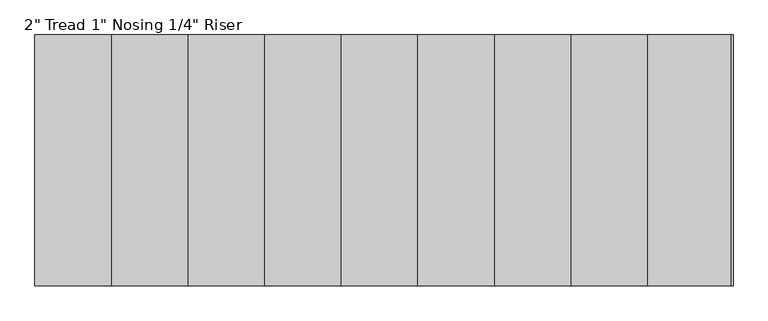
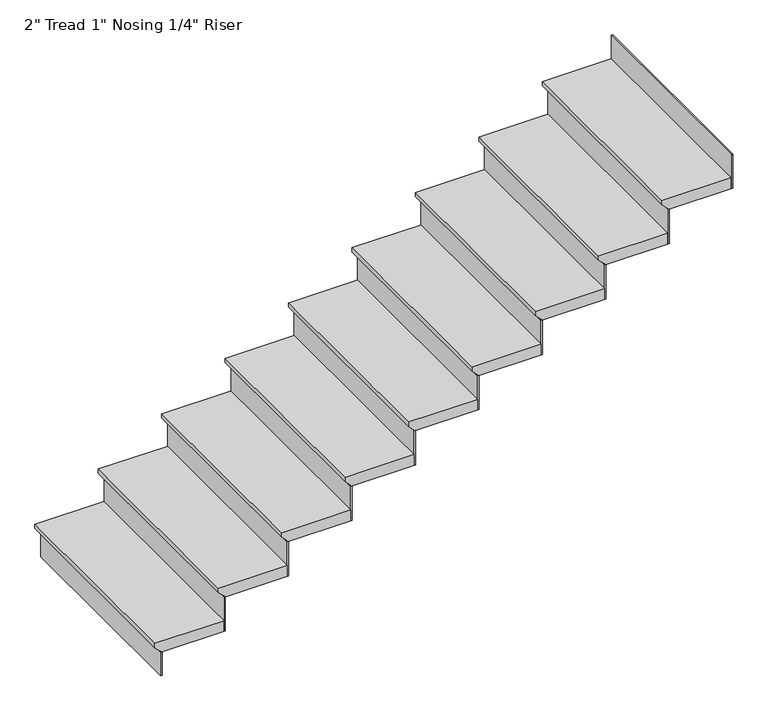
"""IFC4 building model written with IfcOpenShell, lengths in millimetres: stair flight geometry."""

from ifc_helpers import new_model, si_unit, origin, place, context, project, spatial, faceted_brep, source, transform, mapped, element, save


def stair_flight_54a58d27(model_context):
    return source(origin(), model_context, "Body", "Brep", [
        faceted_brep([(-1591.1154463, -4737.3544725, 3341.37), (-1591.1154463, -4737.3544725, 3360.42), (-1591.1154463, -3822.9544725, 3360.42), (-1591.1154463, -3822.9544725, 3341.37), (-1565.7154463, -4737.3544725, 3315.97), (-1565.7154463, -3822.9544725, 3315.97), (-1286.3154463, -4737.3544725, 3360.42), (-1286.3154463, -3822.9544725, 3360.42), (-1565.7154463, -3822.9544725, 3309.62), (-1286.3154463, -3822.9544725, 3309.62), (-1286.3154463, -4737.3544725, 3309.62), (-1565.7154463, -4737.3544725, 3309.62)], [[[0, 1, 2, 3]], [[4, 0, 3, 5]], [[2, 1, 6, 7]], [[8, 9, 10, 11]], [[2, 7, 9, 8, 5, 3]], [[8, 11, 4, 5]], [[6, 1, 0, 4, 11, 10]], [[7, 6, 10, 9]]]),
        faceted_brep([(-1565.7154463, -4737.3544725, 3309.62), (-1565.7154463, -4737.3544725, 3200.4), (-1559.3654463, -4737.3544725, 3200.4), (-1559.3654463, -4737.3544725, 3309.62), (-1565.7154463, -3822.9544725, 3309.62), (-1559.3654463, -3822.9544725, 3309.62), (-1559.3654463, -3822.9544725, 3200.4), (-1565.7154463, -3822.9544725, 3200.4)], [[[0, 1, 2, 3]], [[4, 5, 6, 7]], [[1, 0, 4, 7]], [[2, 1, 7, 6]], [[3, 2, 6, 5]], [[0, 3, 5, 4]]]),
        faceted_brep([(-1286.3154463, -4737.3544725, 3469.64), (-1286.3154463, -4737.3544725, 3309.62), (-1279.9654463, -4737.3544725, 3309.62), (-1279.9654463, -4737.3544725, 3469.64), (-1286.3154463, -3822.9544725, 3469.64), (-1279.9654463, -3822.9544725, 3469.64), (-1279.9654463, -3822.9544725, 3309.62), (-1286.3154463, -3822.9544725, 3309.62)], [[[0, 1, 2, 3]], [[4, 5, 6, 7]], [[1, 0, 4, 7]], [[2, 1, 7, 6]], [[3, 2, 6, 5]], [[0, 3, 5, 4]]]),
        faceted_brep([(-1311.7154463, -3822.9544725, 3520.44), (-1311.7154463, -4737.3544725, 3520.44), (-1006.9154463, -4737.3544725, 3520.44), (-1006.9154463, -3822.9544725, 3520.44), (-1286.3154463, -3822.9544725, 3469.64), (-1006.9154463, -3822.9544725, 3469.64), (-1006.9154463, -4737.3544725, 3469.64), (-1286.3154463, -4737.3544725, 3469.64), (-1286.3154463, -3822.9544725, 3475.99), (-1311.7154463, -3822.9544725, 3501.39), (-1286.3154463, -4737.3544725, 3475.99), (-1311.7154463, -4737.3544725, 3501.39)], [[[0, 1, 2, 3]], [[4, 5, 6, 7]], [[0, 3, 5, 4, 8, 9]], [[4, 7, 10, 8]], [[2, 1, 11, 10, 7, 6]], [[3, 2, 6, 5]], [[11, 1, 0, 9]], [[10, 11, 9, 8]]]),
        faceted_brep([(-1006.9154463, -4737.3544725, 3629.66), (-1006.9154463, -4737.3544725, 3469.64), (-1000.5654463, -4737.3544725, 3469.64), (-1000.5654463, -4737.3544725, 3629.66), (-1006.9154463, -3822.9544725, 3629.66), (-1000.5654463, -3822.9544725, 3629.66), (-1000.5654463, -3822.9544725, 3469.64), (-1006.9154463, -3822.9544725, 3469.64)], [[[0, 1, 2, 3]], [[4, 5, 6, 7]], [[1, 0, 4, 7]], [[2, 1, 7, 6]], [[3, 2, 6, 5]], [[0, 3, 5, 4]]]),
        faceted_brep([(-1032.3154463, -3822.9544725, 3680.46), (-1032.3154463, -4737.3544725, 3680.46), (-727.5154463, -4737.3544725, 3680.46), (-727.5154463, -3822.9544725, 3680.46), (-1006.9154463, -3822.9544725, 3629.66), (-727.5154463, -3822.9544725, 3629.66), (-727.5154463, -4737.3544725, 3629.66), (-1006.9154463, -4737.3544725, 3629.66), (-1006.9154463, -3822.9544725, 3636.01), (-1032.3154463, -3822.9544725, 3661.41), (-1006.9154463, -4737.3544725, 3636.01), (-1032.3154463, -4737.3544725, 3661.41)], [[[0, 1, 2, 3]], [[4, 5, 6, 7]], [[0, 3, 5, 4, 8, 9]], [[4, 7, 10, 8]], [[2, 1, 11, 10, 7, 6]], [[3, 2, 6, 5]], [[11, 1, 0, 9]], [[10, 11, 9, 8]]]),
        faceted_brep([(-727.5154463, -4737.3544725, 3789.68), (-727.5154463, -4737.3544725, 3629.66), (-721.1654463, -4737.3544725, 3629.66), (-721.1654463, -4737.3544725, 3789.68), (-727.5154463, -3822.9544725, 3789.68), (-721.1654463, -3822.9544725, 3789.68), (-721.1654463, -3822.9544725, 3629.66), (-727.5154463, -3822.9544725, 3629.66)], [[[0, 1, 2, 3]], [[4, 5, 6, 7]], [[1, 0, 4, 7]], [[2, 1, 7, 6]], [[3, 2, 6, 5]], [[0, 3, 5, 4]]]),
        faceted_brep([(-752.9154463, -3822.9544725, 3840.48), (-752.9154463, -4737.3544725, 3840.48), (-448.1154463, -4737.3544725, 3840.48), (-448.1154463, -3822.9544725, 3840.48), (-727.5154463, -3822.9544725, 3789.68), (-448.1154463, -3822.9544725, 3789.68), (-448.1154463, -4737.3544725, 3789.68), (-727.5154463, -4737.3544725, 3789.68), (-727.5154463, -3822.9544725, 3796.03), (-752.9154463, -3822.9544725, 3821.43), (-727.5154463, -4737.3544725, 3796.03), (-752.9154463, -4737.3544725, 3821.43)], [[[0, 1, 2, 3]], [[4, 5, 6, 7]], [[0, 3, 5, 4, 8, 9]], [[4, 7, 10, 8]], [[2, 1, 11, 10, 7, 6]], [[3, 2, 6, 5]], [[11, 1, 0, 9]], [[10, 11, 9, 8]]]),
        faceted_brep([(-448.1154463, -4737.3544725, 3949.7), (-448.1154463, -4737.3544725, 3789.68), (-441.7654463, -4737.3544725, 3789.68), (-441.7654463, -4737.3544725, 3949.7), (-448.1154463, -3822.9544725, 3949.7), (-441.7654463, -3822.9544725, 3949.7), (-441.7654463, -3822.9544725, 3789.68), (-448.1154463, -3822.9544725, 3789.68)], [[[0, 1, 2, 3]], [[4, 5, 6, 7]], [[1, 0, 4, 7]], [[2, 1, 7, 6]], [[3, 2, 6, 5]], [[0, 3, 5, 4]]]),
        faceted_brep([(-473.5154463, -3822.9544725, 4000.5), (-473.5154463, -4737.3544725, 4000.5), (-168.7154463, -4737.3544725, 4000.5), (-168.7154463, -3822.9544725, 4000.5), (-448.1154463, -3822.9544725, 3949.7), (-168.7154463, -3822.9544725, 3949.7), (-168.7154463, -4737.3544725, 3949.7), (-448.1154463, -4737.3544725, 3949.7), (-448.1154463, -3822.9544725, 3956.05), (-473.5154463, -3822.9544725, 3981.45), (-448.1154463, -4737.3544725, 3956.05), (-473.5154463, -4737.3544725, 3981.45)], [[[0, 1, 2, 3]], [[4, 5, 6, 7]], [[0, 3, 5, 4, 8, 9]], [[4, 7, 10, 8]], [[2, 1, 11, 10, 7, 6]], [[3, 2, 6, 5]], [[11, 1, 0, 9]], [[10, 11, 9, 8]]]),
        faceted_brep([(-168.7154463, -4737.3544725, 4109.72), (-168.7154463, -4737.3544725, 3949.7), (-162.3654463, -4737.3544725, 3949.7), (-162.3654463, -4737.3544725, 4109.72), (-168.7154463, -3822.9544725, 4109.72), (-162.3654463, -3822.9544725, 4109.72), (-162.3654463, -3822.9544725, 3949.7), (-168.7154463, -3822.9544725, 3949.7)], [[[0, 1, 2, 3]], [[4, 5, 6, 7]], [[1, 0, 4, 7]], [[2, 1, 7, 6]], [[3, 2, 6, 5]], [[0, 3, 5, 4]]]),
        faceted_brep([(-194.1154463, -3822.9544725, 4160.52), (-194.1154463, -4737.3544725, 4160.52), (110.6845537, -4737.3544725, 4160.52), (110.6845537, -3822.9544725, 4160.52), (-168.7154463, -3822.9544725, 4109.72), (110.6845537, -3822.9544725, 4109.72), (110.6845537, -4737.3544725, 4109.72), (-168.7154463, -4737.3544725, 4109.72), (-168.7154463, -3822.9544725, 4116.07), (-194.1154463, -3822.9544725, 4141.47), (-168.7154463, -4737.3544725, 4116.07), (-194.1154463, -4737.3544725, 4141.47)], [[[0, 1, 2, 3]], [[4, 5, 6, 7]], [[0, 3, 5, 4, 8, 9]], [[4, 7, 10, 8]], [[2, 1, 11, 10, 7, 6]], [[3, 2, 6, 5]], [[11, 1, 0, 9]], [[10, 11, 9, 8]]]),
        faceted_brep([(110.6845537, -4737.3544725, 4269.74), (110.6845537, -4737.3544725, 4109.72), (117.0345537, -4737.3544725, 4109.72), (117.0345537, -4737.3544725, 4269.74), (110.6845537, -3822.9544725, 4269.74), (117.0345537, -3822.9544725, 4269.74), (117.0345537, -3822.9544725, 4109.72), (110.6845537, -3822.9544725, 4109.72)], [[[0, 1, 2, 3]], [[4, 5, 6, 7]], [[1, 0, 4, 7]], [[2, 1, 7, 6]], [[3, 2, 6, 5]], [[0, 3, 5, 4]]]),
        faceted_brep([(85.2845537, -3822.9544725, 4320.54), (85.2845537, -4737.3544725, 4320.54), (390.0845537, -4737.3544725, 4320.54), (390.0845537, -3822.9544725, 4320.54), (110.6845537, -3822.9544725, 4269.74), (390.0845537, -3822.9544725, 4269.74), (390.0845537, -4737.3544725, 4269.74), (110.6845537, -4737.3544725, 4269.74), (110.6845537, -3822.9544725, 4276.09), (85.2845537, -3822.9544725, 4301.49), (110.6845537, -4737.3544725, 4276.09), (85.2845537, -4737.3544725, 4301.49)], [[[0, 1, 2, 3]], [[4, 5, 6, 7]], [[0, 3, 5, 4, 8, 9]], [[4, 7, 10, 8]], [[2, 1, 11, 10, 7, 6]], [[3, 2, 6, 5]], [[11, 1, 0, 9]], [[10, 11, 9, 8]]]),
        faceted_brep([(390.0845537, -4737.3544725, 4429.76), (390.0845537, -4737.3544725, 4269.74), (396.4345537, -4737.3544725, 4269.74), (396.4345537, -4737.3544725, 4429.76), (390.0845537, -3822.9544725, 4429.76), (396.4345537, -3822.9544725, 4429.76), (396.4345537, -3822.9544725, 4269.74), (390.0845537, -3822.9544725, 4269.74)], [[[0, 1, 2, 3]], [[4, 5, 6, 7]], [[1, 0, 4, 7]], [[2, 1, 7, 6]], [[3, 2, 6, 5]], [[0, 3, 5, 4]]]),
        faceted_brep([(364.6845537, -3822.9544725, 4480.56), (364.6845537, -4737.3544725, 4480.56), (669.4845537, -4737.3544725, 4480.56), (669.4845537, -3822.9544725, 4480.56), (390.0845537, -3822.9544725, 4429.76), (669.4845537, -3822.9544725, 4429.76), (669.4845537, -4737.3544725, 4429.76), (390.0845537, -4737.3544725, 4429.76), (390.0845537, -3822.9544725, 4436.11), (364.6845537, -3822.9544725, 4461.51), (390.0845537, -4737.3544725, 4436.11), (364.6845537, -4737.3544725, 4461.51)], [[[0, 1, 2, 3]], [[4, 5, 6, 7]], [[0, 3, 5, 4, 8, 9]], [[4, 7, 10, 8]], [[2, 1, 11, 10, 7, 6]], [[3, 2, 6, 5]], [[11, 1, 0, 9]], [[10, 11, 9, 8]]]),
        faceted_brep([(948.8845537, -4737.3544725, 4749.8), (948.8845537, -4737.3544725, 4589.78), (955.2345537, -4737.3544725, 4589.78), (955.2345537, -4737.3544725, 4749.8), (948.8845537, -3822.9544725, 4749.8), (955.2345537, -3822.9544725, 4749.8), (955.2345537, -3822.9544725, 4589.78), (948.8845537, -3822.9544725, 4589.78)], [[[0, 1, 2, 3]], [[4, 5, 6, 7]], [[1, 0, 4, 7]], [[2, 1, 7, 6]], [[3, 2, 6, 5]], [[0, 3, 5, 4]]]),
        faceted_brep([(669.4845537, -4737.3544725, 4589.78), (669.4845537, -4737.3544725, 4429.76), (675.8345537, -4737.3544725, 4429.76), (675.8345537, -4737.3544725, 4589.78), (669.4845537, -3822.9544725, 4589.78), (675.8345537, -3822.9544725, 4589.78), (675.8345537, -3822.9544725, 4429.76), (669.4845537, -3822.9544725, 4429.76)], [[[0, 1, 2, 3]], [[4, 5, 6, 7]], [[1, 0, 4, 7]], [[2, 1, 7, 6]], [[3, 2, 6, 5]], [[0, 3, 5, 4]]]),
        faceted_brep([(948.8845537, -3822.9544725, 4640.58), (923.4845537, -3822.9544725, 4640.58), (644.0845537, -3822.9544725, 4640.58), (644.0845537, -4737.3544725, 4640.58), (948.8845537, -4737.3544725, 4640.58), (923.4845537, -3822.9544725, 4589.78), (948.8845537, -3822.9544725, 4589.78), (948.8845537, -4737.3544725, 4589.78), (669.4845537, -4737.3544725, 4589.78), (669.4845537, -3822.9544725, 4589.78), (669.4845537, -3822.9544725, 4596.13), (644.0845537, -3822.9544725, 4621.53), (669.4845537, -4737.3544725, 4596.13), (644.0845537, -4737.3544725, 4621.53)], [[[0, 1, 2, 3, 4]], [[5, 6, 7, 8, 9]], [[1, 0, 6, 5]], [[2, 1, 5, 9, 10, 11]], [[9, 8, 12, 10]], [[4, 3, 13, 12, 8, 7]], [[0, 4, 7, 6]], [[13, 3, 2, 11]], [[12, 13, 11, 10]]]),
    ])


if __name__ == "__main__":
    model = new_model("IFC4")
    model_context = context("Model", 3, world=origin())
    ifc_project = project(units=[si_unit("LENGTHUNIT", "METRE", prefix="MILLI")], contexts=[model_context])
    site = spatial("IfcSite", under=ifc_project)
    building = spatial("IfcBuilding", under=site)
    placement = place(None, origin())
    stair_flight_shape = stair_flight_54a58d27(model_context)
    element("IfcStairFlight", 1, ObjectType="2\" Tread 1\" Nosing 1/4\" Riser", at=placement, inside=building, context=model_context, shape_type="MappedRepresentation", body=[
        mapped(stair_flight_shape, transform((0.0, 0.0, 0.0), x_axis=(1.0, 0.0, 0.0), y_axis=(0.0, 1.0, 0.0), z_axis=(0.0, 0.0, 1.0))),
    ])
    save(model, "model.ifc")
